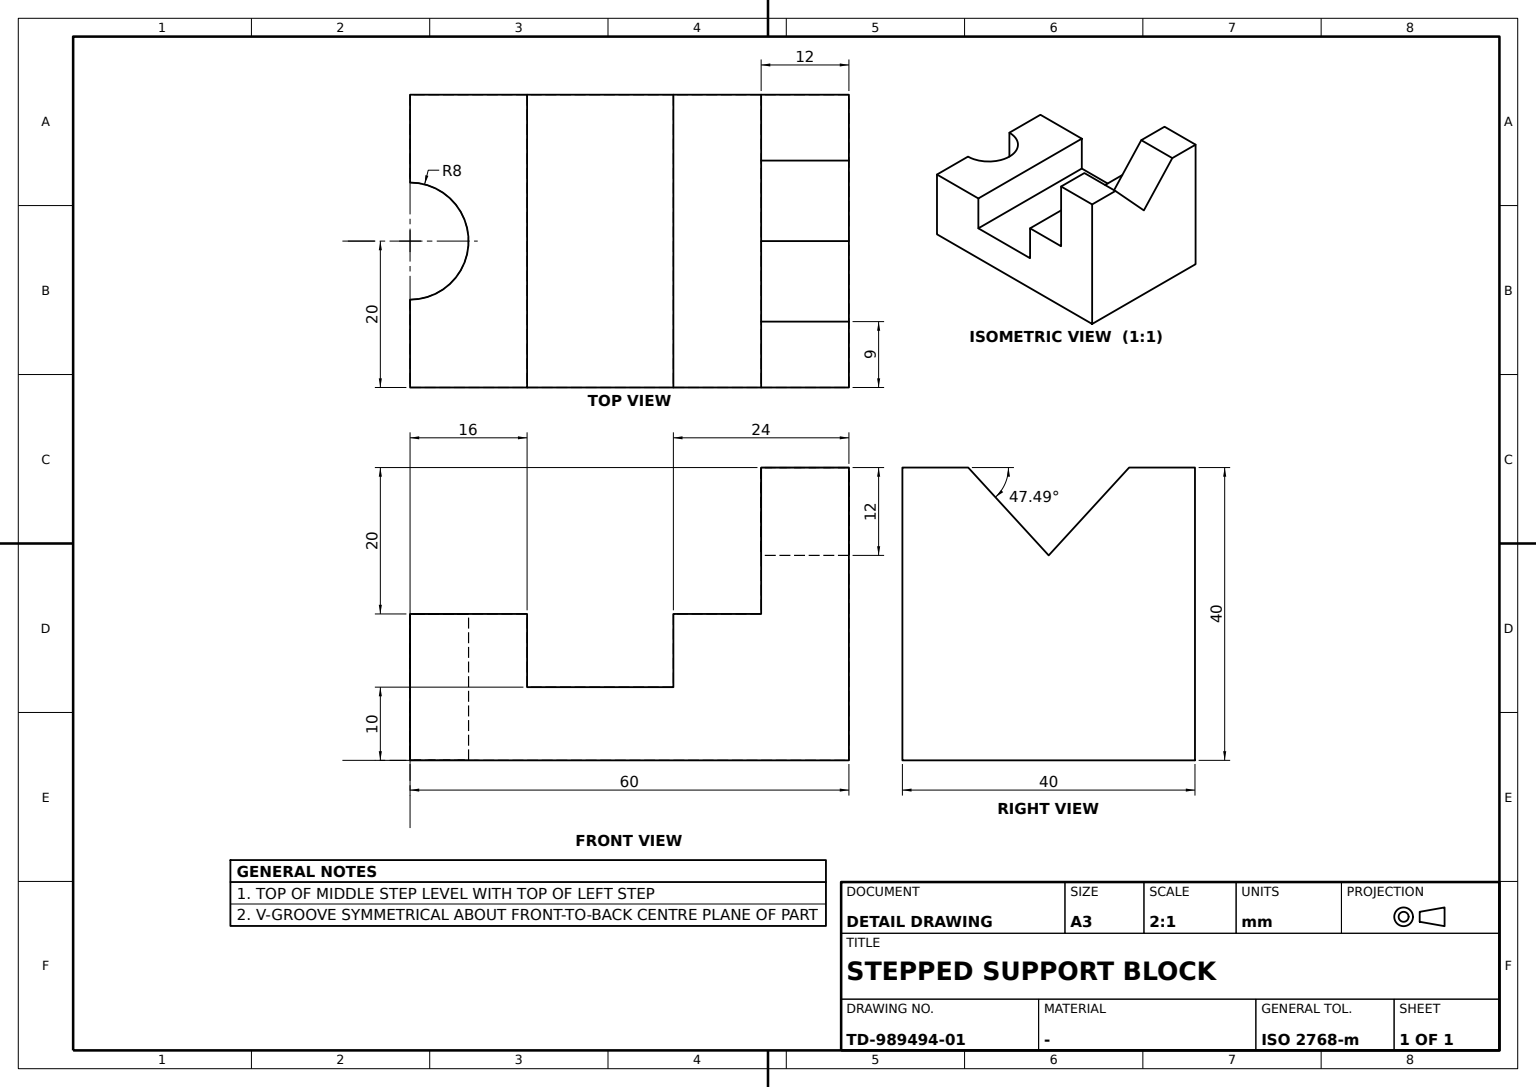
CATIA V5 part; units mm, degrees
sketch "Sketch1" plane through (0, 0, 0) normal (1, 0, 0) x (0, 1, 0)
  line L0 (0, 0) -> (0, 20)
  point P0 (0, 20)
  line L1 (0, 20) -> (16, 20)
  line L2 (16, 20) -> (16, 10)
  line L3 (16, 10) -> (36, 10)
  line L4 (36, 10) -> (36, 20)
  point P1 (36, 20)
  line L5 (36, 20) -> (48, 20)
  line L6 (48, 20) -> (48, 40)
  line L7 (48, 40) -> (60, 40)
  line L8 (60, 40) -> (60, 0)
  point P2 (60, 0)
  line L9 (60, 0) -> (0, 0)
  dimension "length L8" = 40
  dimension "length L7" = 12
  dimension "length L9" = 60
  dimension "length L4" = 10
  dimension "distance L4 L8" = 24
  dimension "length L1" = 16
  dimension "D7" = 20
  constraint vertical L0 y-axis
  constraint vertical L2 y-axis
  constraint vertical L4 y-axis
  constraint vertical L6 y-axis
  constraint vertical L8 y-axis
  constraint horizontal L1 x-axis
  constraint horizontal L3 x-axis
  constraint horizontal L5 x-axis
  constraint horizontal L7 x-axis
  constraint horizontal L9 x-axis
  constraint coincidence P1 L1
  constraint coincidence P2 x-axis
extrude "Pad1" add sketch "Sketch1" along normal mid plane 40
sketch "Sketch2" plane through (0, 60, 0) normal (0, 1, 0) x (-1, 0, 0)
  line L0 (-11, 40) -> (0, 28)
  line L1 (0, 28) -> (11, 40)
  line L2 (-11, 40) -> (11, 40)
  constraint horizontal L2 x-axis
extrude "Pocket1" cut sketch "Sketch2" against normal blind 20
sketch "Sketch3" plane through (0, 0, 20) normal (0, 0, 1) x (1, 0, 0)
  arc A0 (8, 0) -> (-8, 0) centre (0, 0) ccw
  dimension "radius A0" = 8
extrude "Pocket2" cut sketch "Sketch3" against normal up to next material side at (0, 7.95, 20)
properties part number "catia 9"
